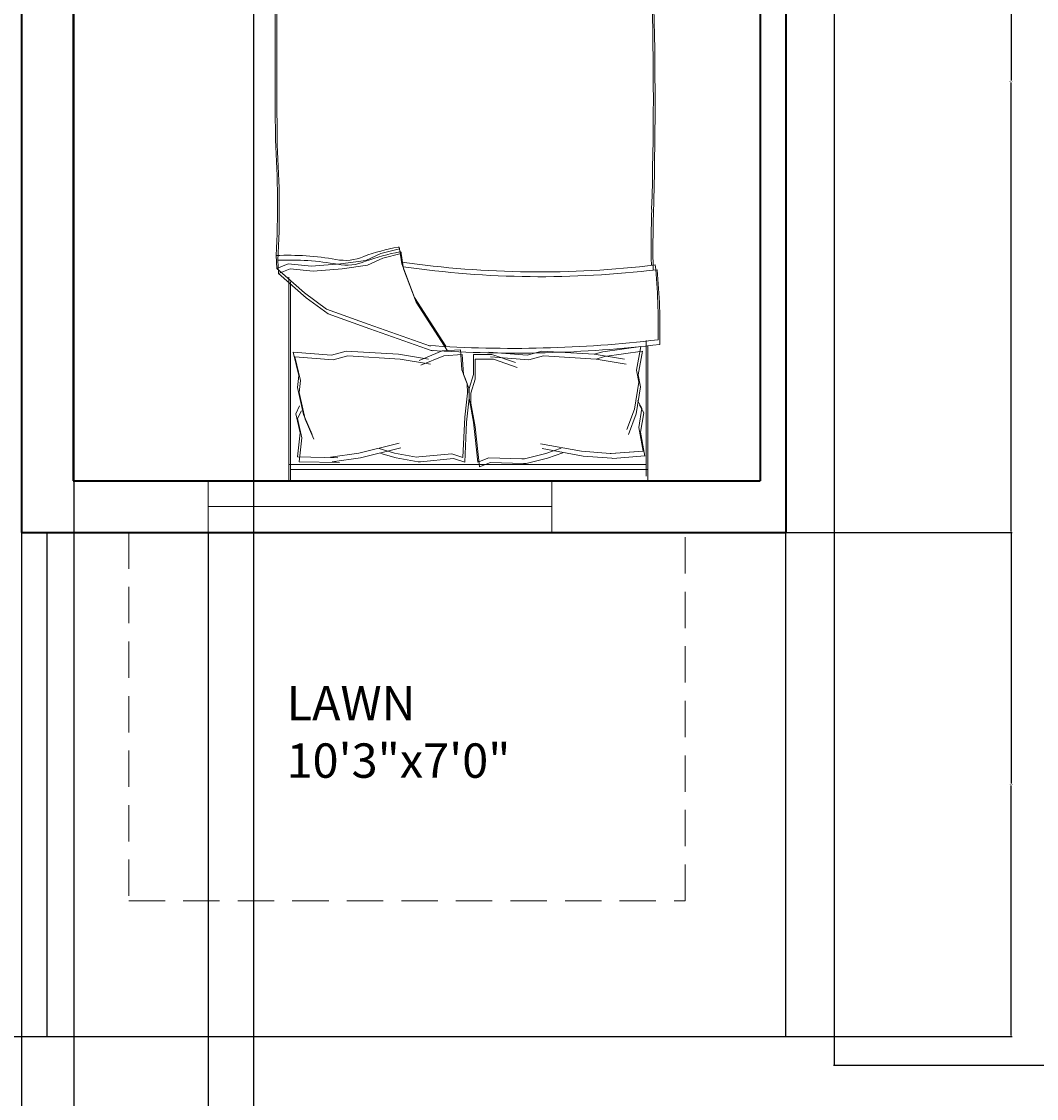
# Model space of a CAD drawing. Units: inches. Extents: x 1734 to 2405, y 1500 to 2491.
# Tile 6 of 14: x 1900 to 2078, y 1700 to 1888. Entities that reach past the tile are written whole.
import ezdxf

# ---------------------------------------------------------------- set-up
doc = ezdxf.new("R2010")
doc.units = ezdxf.units.IN
doc.linetypes.add('DASHED2', pattern=[9.525, 6.35, -3.175])
for name, color, linetype, lineweight in [('A-ANNO-DIMS', 2, 'Continuous', 18), ('A-AREA-IDEN', 7, 'Continuous', 18), ('A-FURN', 8, 'Continuous', 13), ('A-GLAZ', 4, 'Continuous', 18), ('A-WALL', 7, 'Continuous', 35), ('C-PROP', 7, 'Continuous', 25), ('L-PLNT', 3, 'DASHED2', 13)]:
    doc.layers.add(name, color=color, linetype=linetype, lineweight=lineweight)
doc.styles.get("Standard").update_dxf_attribs({"font": 'arial.ttf'})
doc.dimstyles.get("Standard").update_dxf_attribs({"dimtxt": 0.18, "dimasz": 0.18, "dimexe": 0.18, "dimexo": 0.0625, "dimgap": 0.09, "dimtad": 0, "dimtih": 1, "dimtoh": 1, "dimdec": 4, "dimzin": 0, "dimdsep": 46, "dimtxsty": 'Standard', "dimcen": 0.09, "dimadec": 0, "dimazin": 0, "dimtfac": 1, "dimtdec": 4, "dimtofl": 0, "dimtmove": 0, "dimatfit": 3, "dimfxl": 1, "dimtolj": 1, "dimtzin": 0, "dimarcsym": 0})

# ---------------------------------------------------------------- blocks, each defined once
blk = doc.blocks.new('BED-DOUBLE')
for p, q in [((81.88, 67.96), (105.53, 67.96)), ((81.88, 67.96), (105.53, 67.96)), ((82.71, 68.26), (106.37, 68.26)), ((82.71, 68.26), (106.37, 68.26)), ((102.04, 67.71), (97.88, 66.95)), ((102.04, 67.71), (97.88, 66.95)), ((103.53, 67.96), (103.53, 5.54)), ((103.53, 67.96), (103.53, 5.54)), ((104.36, 68.26), (104.36, 5.84)), ((104.36, 68.26), (104.36, 5.84)), ((106.37, 5.54), (106.37, 67.96)), ((83.83, 60.38), (82.88, 67.03)), ((82.88, 67.03), (87.04, 66.28)), ((83.83, 60.38), (82.88, 67.03)), ((82.88, 67.03), (87.04, 66.28)), ((84.66, 60.68), (83.72, 67.33)), ((83.72, 67.33), (87.87, 66.58)), ((84.66, 60.68), (83.72, 67.33)), ((83.72, 67.33), (87.87, 66.58)), ((87.04, 66.28), (89.12, 66.66)), ((87.04, 66.28), (89.12, 66.66)), ((87.87, 66.58), (89.95, 66.95)), ((87.87, 66.58), (89.95, 66.95)), ((89.12, 66.66), (93.84, 65.9)), ((89.12, 66.66), (93.84, 65.9)), ((89.95, 66.95), (94.67, 66.2)), ((89.95, 66.95), (94.67, 66.2)), ((93.65, 67.22), (92.33, 66.47)), ((93.65, 67.22), (92.33, 66.47)), ((94.48, 67.52), (93.16, 66.77)), ((94.48, 67.52), (93.16, 66.77)), ((97.05, 66.66), (93.65, 67.22)), ((97.05, 66.66), (93.65, 67.22)), ((93.84, 65.9), (97.42, 64.58)), ((93.84, 65.9), (97.42, 64.58)), ((97.88, 66.95), (94.48, 67.52)), ((97.88, 66.95), (94.48, 67.52)), ((94.67, 66.2), (98.26, 64.88)), ((94.67, 66.2), (98.26, 64.88)), ((101.2, 67.41), (97.05, 66.66)), ((101.2, 67.41), (97.05, 66.66)), ((101.17, 67.41), (101.6, 61.81)), ((101.17, 67.41), (101.6, 61.82)), ((102.01, 67.7), (102.44, 62.11)), ((102.01, 67.7), (102.44, 62.11)), ((85.12, 64.16), (84.25, 58.9)), ((85.12, 64.16), (84.25, 58.9)), ((85.96, 64.46), (85.09, 59.2)), ((85.96, 64.46), (85.09, 59.2)), ((102.44, 62.11), (102.41, 61.98)), ((102.44, 62.11), (102.41, 61.98)), ((84.25, 58.9), (83.83, 60.38)), ((84.25, 58.9), (83.83, 60.38)), ((85.09, 59.2), (84.66, 60.68)), ((85.09, 59.2), (84.66, 60.68)), ((101.58, 61.68), (101.2, 56.68)), ((101.58, 61.68), (101.2, 56.68)), ((101.6, 61.82), (101.58, 61.68)), ((101.6, 61.81), (101.58, 61.68)), ((102.41, 61.98), (102.04, 56.98)), ((102.41, 61.98), (102.04, 56.98)), ((84.25, 58.9), (83.69, 49.74)), ((84.25, 58.9), (83.69, 49.74)), ((85.09, 59.2), (84.52, 50.04)), ((85.09, 59.2), (84.52, 50.04)), ((101.2, 56.68), (99.88, 49.51)), ((101.2, 56.68), (99.88, 49.51)), ((102.04, 56.98), (100.71, 49.81)), ((102.04, 56.98), (100.71, 49.81)), ((2.04, 52.82), (2.04, 20.68)), ((2.04, 52.82), (2.04, 20.68)), ((2.87, 53.12), (2.87, 20.98)), ((2.87, 53.12), (2.87, 20.98)), ((100.64, 53.1), (101.58, 50.45)), ((100.64, 53.1), (101.58, 50.45)), ((101.47, 53.4), (102.41, 50.75)), ((101.47, 53.39), (102.41, 50.75)), ((83.69, 49.74), (84.42, 47.18)), ((83.69, 49.74), (84.42, 47.18)), ((84.52, 50.04), (85.25, 47.48)), ((84.52, 50.04), (85.25, 47.48)), ((101.58, 50.45), (102.52, 46.68)), ((101.58, 50.45), (102.52, 46.68)), ((102.41, 50.75), (103.36, 46.98)), ((102.41, 50.75), (103.36, 46.98)), ((84.42, 47.18), (83.89, 40.48)), ((84.42, 47.18), (83.89, 40.48)), ((85.25, 47.48), (84.72, 40.78)), ((85.25, 47.48), (84.72, 40.78)), ((85.13, 41.32), (86.55, 45.42)), ((85.13, 41.32), (86.55, 45.42)), ((102.52, 46.26), (102.33, 40.45)), ((102.52, 46.26), (102.33, 40.45)), ((102.52, 46.68), (102.52, 46.26)), ((102.52, 46.68), (102.52, 46.26)), ((103.36, 46.56), (103.17, 40.75)), ((103.36, 46.56), (103.17, 40.75)), ((103.36, 46.98), (103.36, 46.56)), ((103.36, 46.98), (103.36, 46.56)), ((84.29, 41.02), (85.72, 45.13)), ((84.29, 41.02), (85.72, 45.12)), ((84.29, 37.81), (84.29, 41.02)), ((84.29, 37.81), (84.29, 41.02)), ((85.13, 38.11), (85.13, 41.32)), ((85.13, 38.11), (85.13, 41.32)), ((102.33, 40.45), (103.09, 38.56)), ((102.33, 40.45), (103.09, 38.56)), ((103.17, 40.75), (103.92, 38.86)), ((103.17, 40.75), (103.92, 38.86)), ((87.79, 37.81), (84.29, 37.81)), ((87.79, 37.81), (84.29, 37.81)), ((88.63, 38.11), (85.13, 38.11)), ((88.63, 38.11), (85.13, 38.11)), ((90.25, 37.05), (87.79, 37.81)), ((90.25, 37.05), (87.79, 37.81)), ((91.08, 37.35), (88.63, 38.11)), ((91.08, 37.35), (88.63, 38.11)), ((96.1, 37.81), (91.95, 37.05)), ((96.1, 37.81), (91.95, 37.05)), ((96.94, 38.11), (92.78, 37.35)), ((96.94, 38.11), (92.78, 37.35)), ((103.09, 38.56), (96.1, 37.81)), ((103.09, 38.56), (96.1, 37.81)), ((103.92, 38.86), (96.94, 38.11)), ((103.92, 38.86), (96.94, 38.11)), ((86.97, 35.76), (83.47, 35.54)), ((86.97, 35.76), (83.47, 35.54)), ((87.8, 36.06), (84.3, 35.84)), ((87.8, 36.06), (84.3, 35.84)), ((84.3, 35.84), (84.51, 32.63)), ((84.3, 35.84), (84.51, 32.64)), ((89.37, 36.67), (86.97, 35.76)), ((89.37, 36.67), (86.97, 35.76)), ((90.2, 36.96), (87.8, 36.06)), ((90.2, 36.96), (87.8, 36.06)), ((91.06, 36.77), (89.37, 36.67)), ((91.06, 36.77), (89.37, 36.67)), ((91.9, 37.07), (90.2, 36.96)), ((91.9, 37.07), (90.2, 36.96)), ((91.95, 37.05), (90.25, 37.05)), ((91.95, 37.05), (90.25, 37.05)), ((95.26, 36.28), (91.06, 36.77)), ((95.26, 36.28), (91.06, 36.77)), ((92.78, 37.35), (91.08, 37.35)), ((92.78, 37.35), (91.08, 37.35)), ((96.09, 36.57), (91.9, 37.07)), ((96.09, 36.58), (91.9, 37.07)), ((102.28, 35.96), (95.26, 36.28)), ((102.28, 35.96), (95.26, 36.28)), ((103.11, 36.26), (96.09, 36.58)), ((103.11, 36.26), (96.09, 36.57)), ((101.64, 34.03), (102.28, 35.96)), ((101.64, 34.03), (102.28, 35.96)), ((102.48, 34.33), (103.11, 36.26)), ((102.48, 34.33), (103.11, 36.26)), ((83.47, 35.54), (83.67, 32.34)), ((83.47, 35.54), (83.67, 32.34)), ((102.19, 28.24), (101.64, 34.03)), ((102.19, 28.24), (101.64, 34.03)), ((103.03, 28.54), (102.48, 34.33)), ((103.03, 28.54), (102.48, 34.33)), ((82.83, 32.98), (74.35, 27.51)), ((82.83, 32.98), (74.35, 27.51)), ((83.66, 33.28), (75.18, 27.8)), ((83.66, 33.28), (75.18, 27.8)), ((83.67, 32.34), (85.35, 28.33)), ((83.67, 32.34), (85.35, 28.33)), ((84.51, 32.64), (86.18, 28.63)), ((84.51, 32.63), (86.18, 28.62)), ((79, 19.42), (82.83, 30.31)), ((79, 19.41), (82.83, 30.3)), ((79.83, 19.71), (83.66, 30.6)), ((79.83, 19.71), (83.66, 30.6)), ((85.96, 30.27), (85.09, 25)), ((85.96, 30.27), (85.09, 25)), ((85.12, 29.97), (84.25, 24.7)), ((85.12, 29.97), (84.25, 24.7)), ((102.22, 27.83), (102.19, 28.24)), ((102.22, 27.83), (102.19, 28.24)), ((103.05, 28.12), (103.03, 28.54)), ((103.05, 28.12), (103.03, 28.54)), ((74.35, 27.51), (68.49, 25.28)), ((74.35, 27.51), (68.49, 25.28)), ((75.18, 27.8), (69.32, 25.58)), ((75.18, 27.8), (69.32, 25.58)), ((101.51, 24), (102.22, 27.83)), ((101.51, 24), (102.22, 27.83)), ((102.35, 24.3), (103.05, 28.12)), ((102.35, 24.3), (103.05, 28.12)), ((68.49, 25.28), (65.86, 24.88)), ((68.49, 25.28), (65.86, 24.88)), ((65.86, 24.88), (66.67, 21.64)), ((65.86, 24.88), (66.67, 21.64)), ((69.32, 25.58), (66.69, 25.17)), ((69.32, 25.58), (66.69, 25.17)), ((66.69, 25.17), (67.5, 21.94)), ((66.69, 25.17), (67.5, 21.94)), ((84.25, 24.7), (83.69, 15.55)), ((84.25, 24.7), (83.69, 15.55)), ((85.09, 25), (84.52, 15.84)), ((85.09, 25), (84.52, 15.85)), ((101.52, 17.76), (99.76, 24.83)), ((101.52, 17.76), (99.76, 24.83)), ((102.36, 18.05), (100.59, 25.13)), ((102.36, 18.05), (100.59, 25.13)), ((100.73, 21.3), (101.51, 24)), ((100.73, 21.3), (101.51, 24)), ((101.57, 21.6), (102.35, 24.3)), ((101.57, 21.6), (102.35, 24.3)), ((66.67, 21.64), (67.88, 19.01)), ((66.67, 21.64), (67.88, 19.01)), ((67.5, 21.94), (68.72, 19.31)), ((67.5, 21.94), (68.72, 19.31)), ((67.88, 19.01), (68.49, 14.56)), ((67.88, 19.01), (68.49, 14.56)), ((68.72, 19.31), (69.32, 14.86)), ((68.72, 19.31), (69.32, 14.86)), ((76.37, 12.13), (79, 19.42)), ((76.37, 12.13), (79, 19.41)), ((77.21, 12.43), (79.83, 19.71)), ((77.21, 12.43), (79.83, 19.71)), ((102.21, 12.8), (101.52, 17.76)), ((102.21, 12.8), (101.52, 17.76)), ((103.05, 13.09), (102.36, 18.05)), ((103.05, 13.09), (102.36, 18.05)), ((83.69, 15.55), (84.42, 12.99)), ((83.69, 15.55), (84.42, 12.99)), ((84.52, 15.85), (85.25, 13.28)), ((84.52, 15.84), (85.25, 13.28)), ((68.49, 14.56), (68.89, 9.5)), ((68.49, 14.56), (68.89, 9.5)), ((69.32, 14.86), (69.73, 9.8)), ((69.32, 14.86), (69.73, 9.8)), ((85.25, 13.28), (84.72, 6.58)), ((85.25, 13.28), (84.72, 6.58)), ((102.19, 7.05), (102.32, 14.11)), ((102.19, 7.05), (102.32, 14.11)), ((102.32, 14.11), (102.21, 12.8)), ((102.32, 14.11), (102.21, 12.8)), ((103.03, 7.35), (103.15, 14.4)), ((103.03, 7.35), (103.15, 14.4)), ((103.15, 14.4), (103.05, 13.09)), ((103.15, 14.4), (103.05, 13.09)), ((73.54, 8.29), (76.37, 12.13)), ((73.54, 8.29), (76.37, 12.13)), ((74.38, 8.59), (77.21, 12.43)), ((74.38, 8.59), (77.21, 12.43)), ((84.42, 12.99), (83.89, 6.28)), ((84.42, 12.99), (83.89, 6.28)), ((68.89, 9.5), (68.49, 5.46)), ((68.89, 9.5), (68.49, 5.46)), ((69.73, 9.8), (69.32, 5.76)), ((69.73, 9.8), (69.32, 5.76)), ((94.75, 8.1), (98.25, 9.64)), ((94.75, 8.1), (98.25, 9.64)), ((95.58, 8.4), (99.08, 9.94)), ((95.58, 8.4), (99.08, 9.94)), ((69.3, 3.45), (73.54, 8.29)), ((69.3, 3.45), (73.54, 8.29)), ((70.13, 3.75), (74.38, 8.59)), ((70.13, 3.75), (74.38, 8.59)), ((84.72, 6.58), (88.82, 7.6)), ((84.72, 6.58), (88.82, 7.59)), ((88.82, 7.6), (90.92, 7.35)), ((88.82, 7.59), (90.92, 7.35)), ((90.08, 7.05), (94.75, 8.1)), ((90.08, 7.05), (94.75, 8.1)), ((90.92, 7.35), (95.58, 8.4)), ((90.92, 7.35), (95.58, 8.4)), ((95.48, 7.07), (94.11, 7.74)), ((95.48, 7.07), (94.11, 7.74)), ((98, 7.54), (94.64, 6.77)), ((98, 7.54), (94.64, 6.77)), ((98.83, 7.84), (95.48, 7.07)), ((98.83, 7.84), (95.48, 7.07)), ((102.19, 7.05), (98, 7.54)), ((102.19, 7.05), (98, 7.54)), ((103.03, 7.35), (98.83, 7.84)), ((103.03, 7.35), (98.83, 7.84)), ((69.32, 5.76), (70.13, 3.75)), ((69.32, 5.76), (70.13, 3.75)), ((106.37, 5.84), (71.61, 5.84)), ((106.37, 5.84), (71.61, 5.84)), ((83.89, 6.28), (87.99, 7.3)), ((83.89, 6.28), (87.99, 7.3)), ((87.99, 7.3), (90.08, 7.05)), ((87.99, 7.3), (90.08, 7.05)), ((94.64, 6.77), (93.28, 7.44)), ((94.64, 6.77), (93.28, 7.44)), ((68.49, 5.46), (69.3, 3.45)), ((68.49, 5.46), (69.3, 3.45)), ((105.53, 5.54), (70.78, 5.54)), ((105.53, 5.54), (70.78, 5.54)), ((106.37, 5.54), (105.53, 5.54)), ((67.02, 3.35), (69.3, 3.45, 5.06)), ((67.02, 3.35), (69.3, 3.45, 5.06)), ((67.85, 3.65), (70.13, 3.75, 5.06)), ((67.85, 3.65), (70.13, 3.75, 5.06))]:
    blk.add_line(p, q)
for centre, radius, start, end in [((1.42, 71.08), 1.42, 56.1736, 203.4781), ((1.42, 71.08), 1.42, 56.1736, 203.4781), ((2.25, 71.38), 1.42, 56.1736, 203.4781), ((2.25, 71.38), 1.42, 56.1736, 203.4781), ((13.75, 100.79), 30.77, 247.9751, 266.652), ((13.75, 100.79), 30.77, 247.9751, 266.652), ((14.58, 101.08), 30.77, 247.9751, 266.652), ((14.58, 101.08), 30.77, 247.9751, 266.652), ((-156.77, 44.51), 159.02, 2.9958, 9.4091), ((-156.77, 44.51), 159.02, 2.9958, 9.4091), ((-155.93, 44.81), 159.02, 2.9958, 9.4091), ((-155.93, 44.81), 159.02, 2.9958, 9.4091), ((21.27, 107.63), 38.7, 256.0648, 268.9113), ((21.27, 107.63), 38.7, 256.0648, 268.9113), ((22.11, 107.93), 38.7, 256.0648, 268.9113), ((22.11, 107.93), 38.7, 256.0648, 268.9113), ((79.29, -38.73), 108.8, 88.7218, 95.604), ((79.29, -38.73), 108.8, 88.7218, 95.604), ((-97.79, 49.61), 168.5, 351.7845, 6.9006), ((-97.79, 49.61), 168.5, 351.7845, 6.9006), ((80.12, -38.43), 108.8, 88.7218, 95.604), ((80.12, -38.43), 108.8, 88.7218, 95.604), ((-132.23, 44.6), 215.46, 356.0865, 6.7821), ((-132.23, 44.6), 215.46, 356.0865, 6.7821), ((-131.4, 44.9), 215.46, 356.0865, 6.7821), ((-131.4, 44.9), 215.46, 356.0865, 6.7821), ((39.43, -560.7), 629.91, 88.22771, 91.71854), ((39.43, -560.7), 629.91, 88.22771, 91.71854), ((40.26, -560.4), 629.91, 88.22771, 91.71854), ((40.26, -560.4), 629.91, 88.22771, 91.71854), ((64.82, 291.01), 222.17, 268.4762, 271.0082), ((64.82, 291.01), 222.17, 268.4762, 271.0082), ((65.65, 291.31), 222.17, 268.4762, 271.0082), ((65.65, 291.31), 222.17, 268.4762, 271.0082), ((-98.62, 49.31), 168.5, 351.7845, 6.9006), ((-98.62, 49.31), 168.5, 351.7845, 6.9006), ((136.5, 94.99), 139.04, 193.3832, 197.7053), ((136.5, 94.99), 139.04, 193.3832, 197.7053), ((137.34, 95.29), 139.04, 193.3832, 197.7053), ((137.34, 95.29), 139.04, 193.3832, 197.7053), ((65.78, 24.65), 0.241, 70.2464, 181.1377), ((65.78, 24.65), 0.241, 70.2464, 181.1377), ((103.6, 31.81), 38.73, 190.6617, 199.8806), ((103.6, 31.81), 38.73, 190.6617, 199.8806), ((66.61, 24.95), 0.241, 70.2464, 181.1377), ((66.61, 24.95), 0.241, 70.2464, 181.1377), ((104.43, 32.11), 38.73, 190.6617, 199.8806), ((104.43, 32.11), 38.73, 190.6617, 199.8806), ((-170.87, 19.05), 173.75, 354.4998, 0.6351), ((-170.87, 19.05), 173.75, 354.4998, 0.6351), ((-171.71, 18.75), 173.75, 354.4998, 0.6351), ((-171.71, 18.75), 173.75, 354.4998, 0.6351), ((60.57, 15.67), 8.13, 348.6608, 23.7384), ((60.57, 15.67), 8.13, 348.6608, 23.7384), ((59.73, 15.37), 8.13, 348.6608, 23.7384), ((59.73, 15.37), 8.13, 348.6608, 23.7384), ((114.23, 5.46), 47.26, 169.8763, 182.5657), ((114.23, 5.46), 47.26, 169.8763, 182.5657), ((115.06, 5.76), 47.26, 169.8763, 182.5657), ((115.06, 5.76), 47.26, 169.8763, 182.5657), ((58.94, -165.25), 169.13, 86.9791, 93.8365), ((58.94, -165.25), 169.13, 86.9791, 93.8365), ((2.53, 1.44), 1.44, 152.6588, 266.02), ((2.53, 1.44), 1.44, 152.6588, 266.02), ((3.36, 1.73), 1.44, 152.6588, 266.02), ((3.36, 1.74), 1.44, 152.6588, 266.02), ((15.85, -26.97), 30.12, 87.4714, 116.4681), ((15.85, -26.97), 30.12, 87.4714, 116.4681), ((16.69, -26.67), 30.12, 87.4714, 116.4681), ((16.69, -26.67), 30.12, 87.4714, 116.4681), ((16.96, 5961.08), 5957.95, 270.002168, 270.286887), ((16.96, 5961.08), 5957.95, 270.002168, 270.286887), ((17.79, 5961.38), 5957.95, 270.002168, 270.286887), ((17.79, 5961.38), 5957.95, 270.002168, 270.286887), ((58.1, -165.55), 169.13, 86.9791, 93.8365), ((58.1, -165.55), 169.13, 86.9791, 93.8365)]:
    blk.add_arc(centre, radius, start, end)
blk = doc.blocks.new('WIN-60-DEEP')
for p, q in [((0, 9), (0, 0)), ((60, 4.5), (60, 9)), ((60, 9), (60, 0)), ((0, 0), (0, 4.5)), ((0, 4.5), (60, 4.5))]:
    blk.add_line(p, q)
blk = doc.blocks.new('*D25')
at = {"layer": 'A-ANNO-DIMS', "color": 0, "lineweight": -2, "transparency": 16777216}
for p, q in [((2033.96, 1798.82), (2073.42, 1798.82)), ((2073.24, 1798.64), (2073.24, 1754.98)), ((2073.24, 1710.95), (2073.24, 1754.61)), ((2033.96, 1710.77), (2073.42, 1710.77))]:
    blk.add_line(p, q, dxfattribs=at)
at = {"layer": 'A-ANNO-DIMS', "color": 0, "transparency": 16777216}
for points in [[(2073.21, 1798.64), (2073.27, 1798.64), (2073.24, 1798.82)], [(2073.21, 1710.95), (2073.27, 1710.95), (2073.24, 1710.77)]]:
    blk.add_solid(points, dxfattribs=at)
at = {"layer": 'Defpoints', "color": 0, "transparency": 16777216}
for p in [(2033.89, 1798.82), (2073.24, 1798.82), (2033.89, 1710.77)]:
    blk.add_point(p, dxfattribs=at)
at = {"layer": 'A-ANNO-DIMS', "color": 0, "transparency": 16777216, "insert": (2073.24, 1754.8), "char_height": 0.18, "attachment_point": 5}
blk.add_mtext('\\A1;88.06', dxfattribs=at)
blk = doc.blocks.new('*D26')
at = {"layer": 'A-ANNO-DIMS', "color": 0, "lineweight": -2, "transparency": 16777216}
for p, q in [((1900.39, 1798.76), (1900.39, 1615.47)), ((1932.99, 1798.76), (1932.99, 1615.47)), ((1900.57, 1615.65), (1916.37, 1615.65)), ((1932.81, 1615.65), (1917.02, 1615.65))]:
    blk.add_line(p, q, dxfattribs=at)
at = {"layer": 'A-ANNO-DIMS', "color": 0, "transparency": 16777216}
for points in [[(1900.57, 1615.68), (1900.57, 1615.62), (1900.39, 1615.65)], [(1932.81, 1615.68), (1932.81, 1615.62), (1932.99, 1615.65)]]:
    blk.add_solid(points, dxfattribs=at)
at = {"layer": 'Defpoints', "color": 0, "transparency": 16777216}
for p in [(1900.39, 1798.82), (1932.99, 1798.82), (1932.99, 1615.65)]:
    blk.add_point(p, dxfattribs=at)
at = {"layer": 'A-ANNO-DIMS', "color": 0, "transparency": 16777216, "insert": (1916.69, 1615.65), "char_height": 0.18, "attachment_point": 5}
blk.add_mtext('\\A1;32.6', dxfattribs=at)
blk = doc.blocks.new('*D27')
at = {"layer": 'A-ANNO-DIMS', "color": 0, "lineweight": -2, "transparency": 16777216}
for p, q in [((2029.46, 1956.32), (2073.42, 1956.32)), ((2073.24, 1956.14), (2073.24, 1877.76)), ((2073.24, 1799), (2073.24, 1877.39)), ((2033.96, 1798.82), (2073.42, 1798.82))]:
    blk.add_line(p, q, dxfattribs=at)
at = {"layer": 'A-ANNO-DIMS', "color": 0, "transparency": 16777216}
for points in [[(2073.21, 1956.14), (2073.27, 1956.14), (2073.24, 1956.32)], [(2073.21, 1799), (2073.27, 1799), (2073.24, 1798.82)]]:
    blk.add_solid(points, dxfattribs=at)
at = {"layer": 'Defpoints', "color": 0, "transparency": 16777216}
for p in [(2029.39, 1956.32), (2073.24, 1956.32), (2033.89, 1798.82)]:
    blk.add_point(p, dxfattribs=at)
at = {"layer": 'A-ANNO-DIMS', "color": 0, "transparency": 16777216, "insert": (2073.24, 1877.57), "char_height": 0.18, "attachment_point": 5}
blk.add_mtext('\\A1;157.5', dxfattribs=at)
blk = doc.blocks.new('*D34')
at = {"layer": 'A-ANNO-DIMS', "color": 0, "lineweight": -2, "transparency": 16777216}
for p, q in [((1940.89, 2204.68), (1940.89, 1615.47)), ((1909.52, 2202.26), (1909.52, 1615.47)), ((1909.7, 1615.65), (1924.81, 1615.65)), ((1940.71, 1615.65), (1925.6, 1615.65))]:
    blk.add_line(p, q, dxfattribs=at)
at = {"layer": 'A-ANNO-DIMS', "color": 0, "transparency": 16777216}
for points in [[(1909.7, 1615.68), (1909.7, 1615.62), (1909.52, 1615.65)], [(1940.71, 1615.68), (1940.71, 1615.62), (1940.89, 1615.65)]]:
    blk.add_solid(points, dxfattribs=at)
at = {"layer": 'Defpoints', "color": 0, "transparency": 16777216}
for p in [(1940.89, 2204.75), (1909.52, 2202.32), (1940.89, 1615.65)]:
    blk.add_point(p, dxfattribs=at)
at = {"layer": 'A-ANNO-DIMS', "color": 0, "transparency": 16777216, "insert": (1925.21, 1615.65), "char_height": 0.18, "attachment_point": 5}
blk.add_mtext('\\A1;31.37', dxfattribs=at)
blk = doc.blocks.new('*D36')
at = {"layer": 'A-ANNO-DIMS', "color": 0, "lineweight": -2, "transparency": 16777216}
for p, q in [((2081.68, 2425.82), (2042.21, 2425.82)), ((2042.39, 2425.64), (2042.39, 2065.96)), ((2042.39, 1705.92), (2042.39, 2065.6)), ((2081.68, 1705.74), (2042.21, 1705.74))]:
    blk.add_line(p, q, dxfattribs=at)
at = {"layer": 'A-ANNO-DIMS', "color": 0, "transparency": 16777216}
for points in [[(2042.36, 2425.64), (2042.42, 2425.64), (2042.39, 2425.82)], [(2042.36, 1705.92), (2042.42, 1705.92), (2042.39, 1705.74)]]:
    blk.add_solid(points, dxfattribs=at)
at = {"layer": 'Defpoints', "color": 0, "transparency": 16777216}
for p in [(2042.39, 2425.82), (2081.74, 2425.82), (2081.74, 1705.74)]:
    blk.add_point(p, dxfattribs=at)
at = {"layer": 'A-ANNO-DIMS', "color": 0, "transparency": 16777216, "insert": (2042.39, 2065.78), "char_height": 0.18, "attachment_point": 5}
blk.add_mtext('\\A1;720.1', dxfattribs=at)

msp = doc.modelspace()

# ---------------------------------------------------------------- linework, layer by layer
at = {"layer": 'A-WALL'}
for p, q in [((2033.8942, 2425.8246), (2033.8942, 1798.8246)), ((1900.3942, 1956.3246), (1900.3942, 1798.8246)), ((1909.3942, 1951.8246), (1909.3942, 1807.8246)), ((2029.3942, 1951.8246), (2029.3942, 1807.8246)), ((1909.3942, 1807.8246), (2029.3942, 1807.8246)), ((1900.3942, 1798.8246), (2033.8942, 1798.8246))]:
    msp.add_line(p, q, dxfattribs=at)
at = {"layer": 'C-PROP'}
for p, q in [((1900.3942, 1798.8246), (1900.3942, 1710.7667)), ((1904.8942, 1710.7667), (1904.8942, 1798.8246)), ((2033.8942, 1710.7667), (2033.8942, 1798.8246)), ((1793.8942, 1710.7667), (2033.8942, 1710.7667)), ((1900.3942, 1710.7667), (1904.8942, 1710.7667))]:
    msp.add_line(p, q, dxfattribs=at)
at = {"layer": 'L-PLNT'}
for p, q in [((1919.1115, 1798.8246), (1919.1115, 1798.8246)), ((1919.1115, 1798.8246), (1919.1115, 1734.4878)), ((2016.3206, 1734.4878), (2016.3206, 1798.8246)), ((1919.1115, 1734.4878), (2016.3206, 1734.4878))]:
    msp.add_line(p, q, dxfattribs=at)

# ---------------------------------------------------------------- block references
at = {"layer": 'A-FURN', "rotation": 270}
msp.add_blockref('BED-DOUBLE', (1941.5278, 1914.192), dxfattribs=at)
at = {"layer": 'A-GLAZ'}
msp.add_blockref('WIN-60-DEEP', (1932.992, 1798.825), dxfattribs=at)

# ---------------------------------------------------------------- texts
at = {"layer": 'A-AREA-IDEN', "insert": (1946.6768, 1771.9726), "char_height": 6, "attachment_point": 1}
msp.add_mtext_dynamic_manual_height_columns('LAWN\\P10\'3"x7\'0"', width=110.273273, gutter_width=12.5, heights=[0], dxfattribs=at)

# ---------------------------------------------------------------- dimensions: what is measured, and where the dimension line sits
at = {"layer": 'A-ANNO-DIMS'}
for base, p1, p2, override, picture, middle in [((2042.3945, 2425.8246), (2081.7445, 1705.7415), (2081.7445, 2425.8246), {"dimdec": 1, "dimlfac": 1, "dimrnd": 0, "dimzin": 0, "dimdsep": 46, "dimlunit": 2}, '*D36', (2042.3945, 2065.783)), ((2073.2442, 1956.3246), (2033.8942, 1798.8246), (2029.3942, 1956.3246), {"dimdec": 1, "dimlfac": 1, "dimrnd": 0, "dimzin": 0, "dimdsep": 46, "dimlunit": 2}, '*D27', (2073.2442, 1877.5746)), ((2073.2442, 1798.8246), (2033.8942, 1710.7667), (2033.8942, 1798.8246), {"dimdec": 2, "dimlfac": 1, "dimrnd": 0, "dimzin": 0, "dimdsep": 46, "dimlunit": 2}, '*D25', (2073.2442, 1754.7956))]:
    dim = msp.add_linear_dim(base=base, p1=p1, p2=p2, angle=90, dimstyle='Standard', override=override, dxfattribs=at)
    dim.commit()
    dim.dimension.update_dxf_attribs({"geometry": picture, "text_midpoint": middle})
for base, p1, p2, override, picture, middle in [((1940.8942, 1615.6468), (1909.5222, 2202.3246), (1940.8942, 2204.7456), {"dimdec": 2, "dimlfac": 1, "dimrnd": 0, "dimzin": 0, "dimdsep": 46, "dimlunit": 2}, '*D34', (1925.2082, 1615.6468)), ((1932.9923, 1615.6468), (1900.3942, 1798.8246), (1932.9923, 1798.8246), {"dimdec": 1, "dimlfac": 1, "dimrnd": 0, "dimzin": 0, "dimdsep": 46, "dimlunit": 2}, '*D26', (1916.6932, 1615.6468))]:
    dim = msp.add_linear_dim(base=base, p1=p1, p2=p2, dimstyle='Standard', override=override, dxfattribs=at)
    dim.commit()
    dim.dimension.update_dxf_attribs({"geometry": picture, "text_midpoint": middle})

doc.saveas('drawing.dxf')
